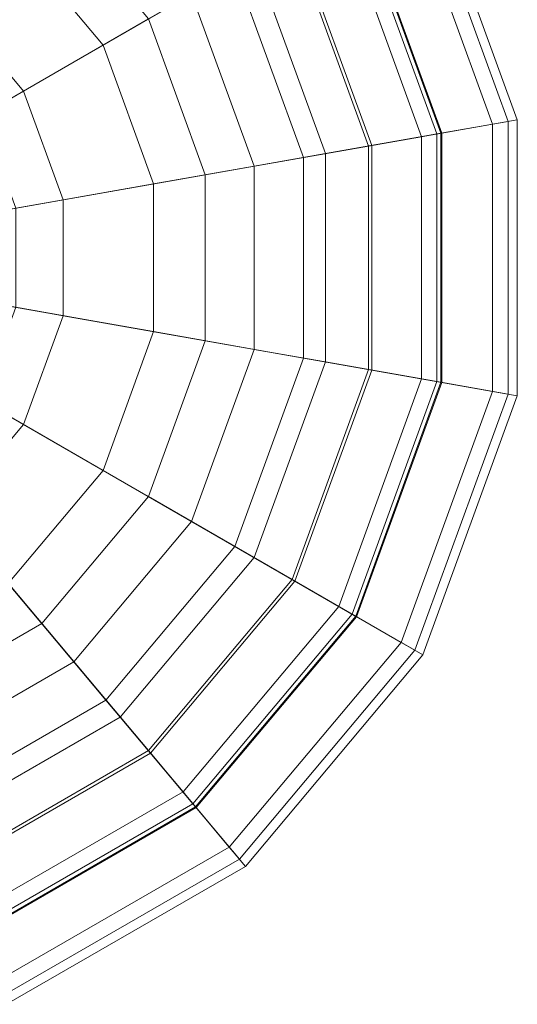
# Model space of a CAD drawing. Units: inches. Extents: x 375 to 1122, y 27 to 1069.
# Tile 49 of 155: x 722.566 to 723.414, y 309.193 to 310.871. Entities that reach past the tile are written whole.
import ezdxf

# ---------------------------------------------------------------- set-up
doc = ezdxf.new("R2010")
doc.units = ezdxf.units.IN
doc.layers.add('Furniture', color=30, linetype='Continuous', lineweight=18)

# ---------------------------------------------------------------- blocks, each defined once
blk = doc.blocks.new('A$C403C54AD')
for points in [[(0.890422, 0.958466, -0.039553), (0.889855, 0.961682, -0.042784), (0.878804, 0.95766, -0.042784), (0.880436, 0.954832, -0.039553)], [(0.889855, 0.961682, -0.042784), (0.895735, 0.928335, -0.039705), (0.895735, 0.928335, -0.039705), (0.878804, 0.95766, -0.042784)], [(0.901048, 0.958466, -0.039553), (0.901615, 0.961682, -0.042784), (0.889855, 0.961682, -0.042784), (0.890422, 0.958466, -0.039553)], [(0.901615, 0.961682, -0.042784), (0.895735, 0.928335, -0.039705), (0.895735, 0.928335, -0.039705), (0.889855, 0.961682, -0.042784)], [(0.912666, 0.95766, -0.042784), (0.895735, 0.928335, -0.039705), (0.895735, 0.928335, -0.039705), (0.901615, 0.961682, -0.042784)], [(0.911033, 0.954832, -0.039553), (0.912666, 0.95766, -0.042784), (0.901615, 0.961682, -0.042784), (0.901048, 0.958466, -0.039553)], [(0.890429, 0.958426, 0.1202), (0.889924, 0.961289, 0.106976), (0.879003, 0.957315, 0.106976), (0.880457, 0.954797, 0.1202)], [(0.889924, 0.961289, 0.106976), (0.890041, 0.960625, 0.078734), (0.87934, 0.95673, 0.078734), (0.879003, 0.957315, 0.106976)], [(0.901041, 0.958426, 0.1202), (0.901545, 0.961289, 0.106976), (0.889924, 0.961289, 0.106976), (0.890429, 0.958426, 0.1202)], [(0.901545, 0.961289, 0.106976), (0.901428, 0.960625, 0.078734), (0.890041, 0.960625, 0.078734), (0.889924, 0.961289, 0.106976)], [(0.911013, 0.954797, 0.1202), (0.912466, 0.957315, 0.106976), (0.901545, 0.961289, 0.106976), (0.901041, 0.958426, 0.1202)], [(0.912466, 0.957315, 0.106976), (0.912129, 0.95673, 0.078734), (0.901428, 0.960625, 0.078734), (0.901545, 0.961289, 0.106976)], [(0.890041, 0.960625, 0.078734), (0.890973, 0.955342, 0.060725), (0.882023, 0.952084, 0.060725), (0.87934, 0.95673, 0.078734)], [(0.901428, 0.960625, 0.078734), (0.900497, 0.955342, 0.060725), (0.890973, 0.955342, 0.060725), (0.890041, 0.960625, 0.078734)], [(0.912129, 0.95673, 0.078734), (0.909447, 0.952084, 0.060725), (0.900497, 0.955342, 0.060725), (0.901428, 0.960625, 0.078734)], [(0.893266, 0.942333, -0.036278), (0.890422, 0.958466, -0.039553), (0.880436, 0.954832, -0.039553), (0.888627, 0.940645, -0.036278)], [(0.891296, 0.953506, 0.129606), (0.890429, 0.958426, 0.1202), (0.880457, 0.954797, 0.1202), (0.882955, 0.95047, 0.129606)], [(0.890459, 0.958252, 0.106759), (0.890947, 0.955485, 0.119395), (0.88195, 0.95221, 0.119395), (0.880545, 0.954643, 0.106759)], [(0.890574, 0.957604, 0.079219), (0.890459, 0.958252, 0.106759), (0.880545, 0.954643, 0.106759), (0.880874, 0.954073, 0.079219)], [(0.898203, 0.942333, -0.036278), (0.901048, 0.958466, -0.039553), (0.890422, 0.958466, -0.039553), (0.893266, 0.942333, -0.036278)], [(0.900173, 0.953506, 0.129606), (0.901041, 0.958426, 0.1202), (0.890429, 0.958426, 0.1202), (0.891296, 0.953506, 0.129606)], [(0.90101, 0.958252, 0.106759), (0.900522, 0.955485, 0.119395), (0.890947, 0.955485, 0.119395), (0.890459, 0.958252, 0.106759)], [(0.900896, 0.957604, 0.079219), (0.90101, 0.958252, 0.106759), (0.890459, 0.958252, 0.106759), (0.890574, 0.957604, 0.079219)], [(0.902842, 0.940645, -0.036278), (0.911033, 0.954832, -0.039553), (0.901048, 0.958466, -0.039553), (0.898203, 0.942333, -0.036278)], [(0.908514, 0.95047, 0.129606), (0.911013, 0.954797, 0.1202), (0.901041, 0.958426, 0.1202), (0.900173, 0.953506, 0.129606)], [(0.910924, 0.954643, 0.106759), (0.909519, 0.95221, 0.119395), (0.900522, 0.955485, 0.119395), (0.90101, 0.958252, 0.106759)], [(0.910595, 0.954073, 0.079219), (0.910924, 0.954643, 0.106759), (0.90101, 0.958252, 0.106759), (0.900896, 0.957604, 0.079219)], [(0.878804, 0.95766, -0.042784), (0.895735, 0.928335, -0.039705), (0.895735, 0.928335, -0.039705), (0.869795, 0.950101, -0.042784)], [(0.891461, 0.952574, 0.062072), (0.890574, 0.957604, 0.079219), (0.880874, 0.954073, 0.079219), (0.883428, 0.94965, 0.062072)], [(0.900009, 0.952574, 0.062072), (0.900896, 0.957604, 0.079219), (0.890574, 0.957604, 0.079219), (0.891461, 0.952574, 0.062072)], [(0.921675, 0.950101, -0.042784), (0.895735, 0.928335, -0.039705), (0.895735, 0.928335, -0.039705), (0.912666, 0.95766, -0.042784)], [(0.908041, 0.94965, 0.062072), (0.910595, 0.954073, 0.079219), (0.900896, 0.957604, 0.079219), (0.900009, 0.952574, 0.062072)], [(0.919142, 0.947976, 0.1202), (0.921369, 0.949844, 0.106976), (0.912466, 0.957315, 0.106976), (0.911013, 0.954797, 0.1202)], [(0.919173, 0.948002, -0.039553), (0.921675, 0.950101, -0.042784), (0.912666, 0.95766, -0.042784), (0.911033, 0.954832, -0.039553)], [(0.921369, 0.949844, 0.106976), (0.920852, 0.949411, 0.078734), (0.912129, 0.95673, 0.078734), (0.912466, 0.957315, 0.106976)], [(0.920852, 0.949411, 0.078734), (0.916743, 0.945962, 0.060725), (0.909447, 0.952084, 0.060725), (0.912129, 0.95673, 0.078734)], [(0.890947, 0.955485, 0.119395), (0.891831, 0.950474, 0.129606), (0.884494, 0.947804, 0.129606), (0.88195, 0.95221, 0.119395)], [(0.890973, 0.955342, 0.060725), (0.8922, 0.948383, 0.050493), (0.885556, 0.945965, 0.050493), (0.882023, 0.952084, 0.060725)], [(0.900522, 0.955485, 0.119395), (0.899638, 0.950474, 0.129606), (0.891831, 0.950474, 0.129606), (0.890947, 0.955485, 0.119395)], [(0.900497, 0.955342, 0.060725), (0.89927, 0.948383, 0.050493), (0.8922, 0.948383, 0.050493), (0.890973, 0.955342, 0.060725)], [(0.909447, 0.952084, 0.060725), (0.905913, 0.945965, 0.050493), (0.89927, 0.948383, 0.050493), (0.900497, 0.955342, 0.060725)], [(0.909519, 0.95221, 0.119395), (0.906975, 0.947804, 0.129606), (0.899638, 0.950474, 0.129606), (0.900522, 0.955485, 0.119395)], [(0.888627, 0.940645, -0.036278), (0.880436, 0.954832, -0.039553), (0.872296, 0.948002, -0.039553), (0.884846, 0.937471, -0.036278)], [(0.906623, 0.937471, -0.036278), (0.919173, 0.948002, -0.039553), (0.911033, 0.954832, -0.039553), (0.902842, 0.940645, -0.036278)], [(0.915314, 0.944764, 0.129606), (0.919142, 0.947976, 0.1202), (0.911013, 0.954797, 0.1202), (0.908514, 0.95047, 0.129606)], [(0.919006, 0.947862, 0.106759), (0.916854, 0.946056, 0.119395), (0.909519, 0.95221, 0.119395), (0.910924, 0.954643, 0.106759)], [(0.918502, 0.947439, 0.079219), (0.919006, 0.947862, 0.106759), (0.910924, 0.954643, 0.106759), (0.910595, 0.954073, 0.079219)], [(0.914589, 0.944156, 0.062072), (0.918502, 0.947439, 0.079219), (0.910595, 0.954073, 0.079219), (0.908041, 0.94965, 0.062072)], [(0.891831, 0.950474, 0.129606), (0.891296, 0.953506, 0.129606), (0.882955, 0.95047, 0.129606), (0.884494, 0.947804, 0.129606)], [(0.899638, 0.950474, 0.129606), (0.900173, 0.953506, 0.129606), (0.891296, 0.953506, 0.129606), (0.891831, 0.950474, 0.129606)], [(0.906975, 0.947804, 0.129606), (0.908514, 0.95047, 0.129606), (0.900173, 0.953506, 0.129606), (0.899638, 0.950474, 0.129606)], [(0.892587, 0.946186, 0.05268), (0.891461, 0.952574, 0.062072), (0.883428, 0.94965, 0.062072), (0.886671, 0.944033, 0.05268)], [(0.898882, 0.946186, 0.05268), (0.900009, 0.952574, 0.062072), (0.891461, 0.952574, 0.062072), (0.892587, 0.946186, 0.05268)], [(0.904798, 0.944033, 0.05268), (0.908041, 0.94965, 0.062072), (0.900009, 0.952574, 0.062072), (0.898882, 0.946186, 0.05268)], [(0.916743, 0.945962, 0.060725), (0.911329, 0.94142, 0.050493), (0.905913, 0.945965, 0.050493), (0.909447, 0.952084, 0.060725)], [(0.916854, 0.946056, 0.119395), (0.912956, 0.942785, 0.129606), (0.906975, 0.947804, 0.129606), (0.909519, 0.95221, 0.119395)], [(0.912956, 0.942785, 0.129606), (0.915314, 0.944764, 0.129606), (0.908514, 0.95047, 0.129606), (0.906975, 0.947804, 0.129606)], [(0.869795, 0.950101, -0.042784), (0.895735, 0.928335, -0.039705), (0.895735, 0.928335, -0.039705), (0.863915, 0.939916, -0.042784)], [(0.927555, 0.939916, -0.042784), (0.895735, 0.928335, -0.039705), (0.895735, 0.928335, -0.039705), (0.921675, 0.950101, -0.042784)], [(0.924448, 0.938785, 0.1202), (0.92718, 0.93978, 0.106976), (0.921369, 0.949844, 0.106976), (0.919142, 0.947976, 0.1202)], [(0.924486, 0.938799, -0.039553), (0.927555, 0.939916, -0.042784), (0.921675, 0.950101, -0.042784), (0.919173, 0.948002, -0.039553)], [(0.92718, 0.93978, 0.106976), (0.926546, 0.939549, 0.078734), (0.920852, 0.949411, 0.078734), (0.921369, 0.949844, 0.106976)], [(0.886671, 0.944033, 0.05268), (0.883428, 0.94965, 0.062072), (0.87688, 0.944156, 0.062072), (0.881848, 0.939987, 0.05268)], [(0.909621, 0.939987, 0.05268), (0.914589, 0.944156, 0.062072), (0.908041, 0.94965, 0.062072), (0.904798, 0.944033, 0.05268)], [(0.926546, 0.939549, 0.078734), (0.921505, 0.937714, 0.060725), (0.916743, 0.945962, 0.060725), (0.920852, 0.949411, 0.078734)], [(0.8922, 0.948383, 0.050493), (0.893978, 0.9383, 0.043125), (0.890675, 0.937098, 0.043125), (0.885556, 0.945965, 0.050493)], [(0.89927, 0.948383, 0.050493), (0.897492, 0.9383, 0.043125), (0.893978, 0.9383, 0.043125), (0.8922, 0.948383, 0.050493)], [(0.905913, 0.945965, 0.050493), (0.900794, 0.937098, 0.043125), (0.897492, 0.9383, 0.043125), (0.89927, 0.948383, 0.050493)], [(0.909092, 0.933196, -0.036278), (0.924486, 0.938799, -0.039553), (0.919173, 0.948002, -0.039553), (0.906623, 0.937471, -0.036278)], [(0.919753, 0.937076, 0.129606), (0.924448, 0.938785, 0.1202), (0.919142, 0.947976, 0.1202), (0.915314, 0.944764, 0.129606)], [(0.924281, 0.938725, 0.106759), (0.921641, 0.937764, 0.119395), (0.916854, 0.946056, 0.119395), (0.919006, 0.947862, 0.106759)], [(0.923663, 0.9385, 0.079219), (0.924281, 0.938725, 0.106759), (0.919006, 0.947862, 0.106759), (0.918502, 0.947439, 0.079219)], [(0.918863, 0.936753, 0.062072), (0.923663, 0.9385, 0.079219), (0.918502, 0.947439, 0.079219), (0.914589, 0.944156, 0.062072)], [(0.894188, 0.937103, 0.046044), (0.892587, 0.946186, 0.05268), (0.886671, 0.944033, 0.05268), (0.891283, 0.936046, 0.046044)], [(0.897281, 0.937103, 0.046044), (0.898882, 0.946186, 0.05268), (0.892587, 0.946186, 0.05268), (0.894188, 0.937103, 0.046044)], [(0.900187, 0.936046, 0.046044), (0.904798, 0.944033, 0.05268), (0.898882, 0.946186, 0.05268), (0.897281, 0.937103, 0.046044)], [(0.921641, 0.937764, 0.119395), (0.91686, 0.936024, 0.129606), (0.912956, 0.942785, 0.129606), (0.916854, 0.946056, 0.119395)], [(0.885556, 0.945965, 0.050493), (0.890675, 0.937098, 0.043125), (0.887983, 0.934839, 0.043125), (0.88014, 0.94142, 0.050493)], [(0.911329, 0.94142, 0.050493), (0.903486, 0.934839, 0.043125), (0.900794, 0.937098, 0.043125), (0.905913, 0.945965, 0.050493)], [(0.921505, 0.937714, 0.060725), (0.914864, 0.935297, 0.050493), (0.911329, 0.94142, 0.050493), (0.916743, 0.945962, 0.060725)], [(0.91686, 0.936024, 0.129606), (0.919753, 0.937076, 0.129606), (0.915314, 0.944764, 0.129606), (0.912956, 0.942785, 0.129606)], [(0.891283, 0.936046, 0.046044), (0.886671, 0.944033, 0.05268), (0.881848, 0.939987, 0.05268), (0.888914, 0.934058, 0.046044)], [(0.902556, 0.934058, 0.046044), (0.909621, 0.939987, 0.05268), (0.904798, 0.944033, 0.05268), (0.900187, 0.936046, 0.046044)], [(0.912769, 0.934534, 0.05268), (0.918863, 0.936753, 0.062072), (0.914589, 0.944156, 0.062072), (0.909621, 0.939987, 0.05268)], [(0.893622, 0.940316, -0.033413), (0.893266, 0.942333, -0.036278), (0.888627, 0.940645, -0.036278), (0.889651, 0.938871, -0.033413)], [(0.897847, 0.940316, -0.033413), (0.898203, 0.942333, -0.036278), (0.893266, 0.942333, -0.036278), (0.893622, 0.940316, -0.033413)], [(0.901818, 0.938871, -0.033413), (0.902842, 0.940645, -0.036278), (0.898203, 0.942333, -0.036278), (0.897847, 0.940316, -0.033413)], [(0.88014, 0.94142, 0.050493), (0.887983, 0.934839, 0.043125), (0.886226, 0.931795, 0.043125), (0.876605, 0.935297, 0.050493)], [(0.914864, 0.935297, 0.050493), (0.905243, 0.931795, 0.043125), (0.903486, 0.934839, 0.043125), (0.911329, 0.94142, 0.050493)], [(0.889651, 0.938871, -0.033413), (0.888627, 0.940645, -0.036278), (0.884846, 0.937471, -0.036278), (0.886415, 0.936155, -0.033413)], [(0.905055, 0.936155, -0.033413), (0.906623, 0.937471, -0.036278), (0.902842, 0.940645, -0.036278), (0.901818, 0.938871, -0.033413)]]:
    blk.add_3dface(points)

msp = doc.modelspace()

# ---------------------------------------------------------------- block references
at = {"layer": 'Furniture', "xscale": 39.9918517141215, "yscale": 39.9918517141215, "zscale": 39.9918517141215, "rotation": 270}
msp.add_blockref('A$C403C54AD', (684.9549, 346.2875, 0.024), dxfattribs=at)

doc.saveas('drawing.dxf')
